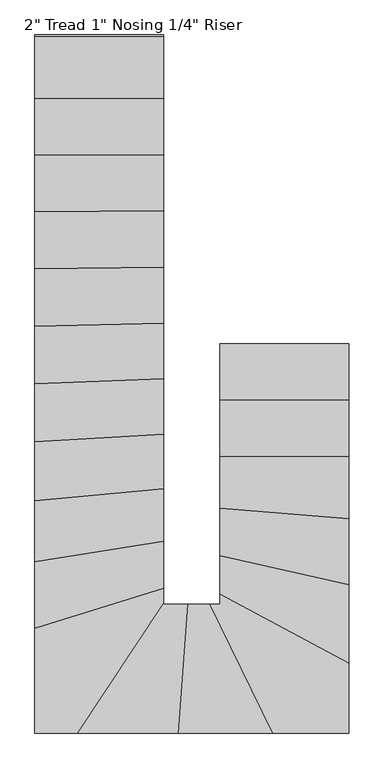
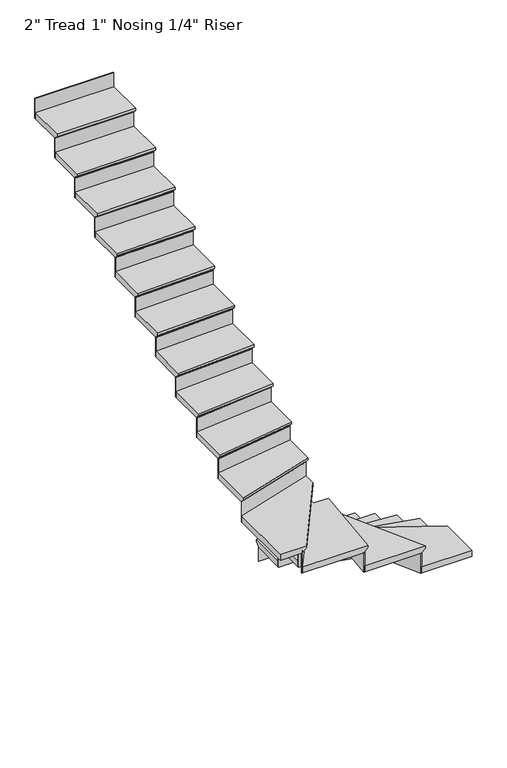
"""IFC4 building model written with IfcOpenShell, lengths in millimetres: stair flight geometry."""

from ifc_helpers import new_model, si_unit, origin, place, context, project, spatial, faceted_brep, source, transform, mapped, element, save


def stair_flight_e7e63c14(model_context):
    return source(origin(), model_context, "Body", "Brep", [
        faceted_brep([(-11643.709927, 2021.0747681, 150.2833333), (-11643.709927, 2021.0747681, 169.3333333), (-11008.709927, 2021.0747681, 169.3333333), (-11008.709927, 2021.0747681, 150.2833333), (-11643.709927, 1995.6747681, 124.8833333), (-11008.709927, 1995.6747681, 124.8833333), (-11643.709927, 1716.2747681, 169.3333333), (-11008.709927, 1716.2747681, 169.3333333), (-11008.709927, 1995.6747681, 118.5333333), (-11008.709927, 1716.2747681, 118.5333333), (-11643.709927, 1716.2747681, 118.5333333), (-11643.709927, 1995.6747681, 118.5333333)], [[[0, 1, 2, 3]], [[4, 0, 3, 5]], [[2, 1, 6, 7]], [[8, 9, 10, 11]], [[2, 7, 9, 8, 5, 3]], [[8, 11, 4, 5]], [[6, 1, 0, 4, 11, 10]], [[7, 6, 10, 9]]]),
        faceted_brep([(-11643.709927, 1995.6747681, 118.5333333), (-11643.709927, 1995.6747681, 0.0), (-11643.709927, 1989.3247681, 0.0), (-11643.709927, 1989.3247681, 118.5333333), (-11008.709927, 1995.6747681, 118.5333333), (-11008.709927, 1989.3247681, 118.5333333), (-11008.709927, 1989.3247681, 0.0), (-11008.709927, 1995.6747681, 0.0)], [[[0, 1, 2, 3]], [[4, 5, 6, 7]], [[1, 0, 4, 7]], [[2, 1, 7, 6]], [[3, 2, 6, 5]], [[0, 3, 5, 4]]]),
        faceted_brep([(-11643.709927, 1716.2747681, 287.8666667), (-11643.709927, 1716.2747681, 118.5333333), (-11643.709927, 1709.9247681, 118.5333333), (-11643.709927, 1709.9247681, 287.8666667), (-11008.709927, 1716.2747681, 287.8666667), (-11008.709927, 1709.9247681, 287.8666667), (-11008.709927, 1709.9247681, 118.5333333), (-11008.709927, 1716.2747681, 118.5333333)], [[[0, 1, 2, 3]], [[4, 5, 6, 7]], [[1, 0, 4, 7]], [[2, 1, 7, 6]], [[3, 2, 6, 5]], [[0, 3, 5, 4]]]),
        faceted_brep([(-11008.709927, 1741.6747681, 338.6666667), (-11643.709927, 1741.6747681, 338.6666667), (-11643.709927, 1436.8747681, 338.6666667), (-11008.709927, 1436.8747681, 338.6666667), (-11008.709927, 1716.2747681, 287.8666667), (-11008.709927, 1436.8747681, 287.8666667), (-11643.709927, 1436.8747681, 287.8666667), (-11643.709927, 1716.2747681, 287.8666667), (-11008.709927, 1716.2747681, 294.2166667), (-11008.709927, 1741.6747681, 319.6166667), (-11643.709927, 1716.2747681, 294.2166667), (-11643.709927, 1741.6747681, 319.6166667)], [[[0, 1, 2, 3]], [[4, 5, 6, 7]], [[0, 3, 5, 4, 8, 9]], [[4, 7, 10, 8]], [[2, 1, 11, 10, 7, 6]], [[3, 2, 6, 5]], [[11, 1, 0, 9]], [[10, 11, 9, 8]]]),
        faceted_brep([(-11643.709927, 1436.8747681, 457.2), (-11643.709927, 1436.8747681, 287.8666667), (-11643.709927, 1430.5247681, 287.8666667), (-11643.709927, 1430.5247681, 457.2), (-11008.709927, 1436.8747681, 457.2), (-11008.709927, 1430.5247681, 457.2), (-11008.709927, 1430.5247681, 287.8666667), (-11008.709927, 1436.8747681, 287.8666667)], [[[0, 1, 2, 3]], [[4, 5, 6, 7]], [[1, 0, 4, 7]], [[2, 1, 7, 6]], [[3, 2, 6, 5]], [[0, 3, 5, 4]]]),
        faceted_brep([(-11008.709927, 1462.2747681, 508.0), (-11643.709927, 1462.2747681, 508.0), (-11643.709927, 1184.2060512, 508.0), (-11008.709927, 1130.5625394, 508.0), (-11008.709927, 1436.8747681, 457.2), (-11008.709927, 1130.5625394, 457.2), (-11643.709927, 1184.2060512, 457.2), (-11643.709927, 1436.8747681, 457.2), (-11008.709927, 1436.8747681, 463.55), (-11008.709927, 1462.2747681, 488.95), (-11643.709927, 1436.8747681, 463.55), (-11643.709927, 1462.2747681, 488.95)], [[[0, 1, 2, 3]], [[4, 5, 6, 7]], [[0, 3, 5, 4, 8, 9]], [[4, 7, 10, 8]], [[2, 1, 11, 10, 7, 6]], [[3, 2, 6, 5]], [[11, 1, 0, 9]], [[10, 11, 9, 8]]]),
        faceted_brep([(-11643.709927, 1184.2060512, 626.5333333), (-11643.709927, 1184.2060512, 457.2), (-11643.709927, 1177.833433, 457.2), (-11643.709927, 1177.833433, 626.5333333), (-11008.709927, 1130.5625394, 626.5333333), (-11008.709927, 1124.1899212, 626.5333333), (-11008.709927, 1124.1899212, 457.2), (-11008.709927, 1130.5625394, 457.2)], [[[0, 1, 2, 3]], [[4, 5, 6, 7]], [[1, 0, 4, 7]], [[2, 1, 7, 6]], [[3, 2, 6, 5]], [[0, 3, 5, 4]]]),
        faceted_brep([(-11008.709927, 1156.0530121, 677.3333333), (-11643.709927, 1209.696524, 677.3333333), (-11643.709927, 949.9239217, 677.3333333), (-11008.709927, 804.9179267, 677.3333333), (-11008.709927, 1130.5625394, 626.5333333), (-11008.709927, 804.9179267, 626.5333333), (-11643.709927, 949.9239217, 626.5333333), (-11643.709927, 1184.2060512, 626.5333333), (-11008.709927, 1130.5625394, 632.8833333), (-11008.709927, 1156.0530121, 658.2833333), (-11643.709927, 1184.2060512, 632.8833333), (-11643.709927, 1209.696524, 658.2833333)], [[[0, 1, 2, 3]], [[4, 5, 6, 7]], [[0, 3, 5, 4, 8, 9]], [[4, 7, 10, 8]], [[2, 1, 11, 10, 7, 6]], [[3, 2, 6, 5]], [[11, 1, 0, 9]], [[10, 11, 9, 8]]]),
        faceted_brep([(-11643.709927, 949.9239217, 795.8666667), (-11643.709927, 949.9239217, 626.5333333), (-11643.709927, 943.4104607, 626.5333333), (-11643.709927, 943.4104607, 795.8666667), (-11008.709927, 804.9179267, 795.8666667), (-11008.709927, 798.4044657, 795.8666667), (-11008.709927, 798.4044657, 626.5333333), (-11008.709927, 804.9179267, 626.5333333)], [[[0, 1, 2, 3]], [[4, 5, 6, 7]], [[1, 0, 4, 7]], [[2, 1, 7, 6]], [[3, 2, 6, 5]], [[0, 3, 5, 4]]]),
        faceted_brep([(-11008.709927, 830.9717706, 846.6666667), (-11643.709927, 975.9777656, 846.6666667), (-11643.709927, 755.0123184, 846.6666667), (-11008.709927, 415.579537, 846.6666667), (-11008.709927, 804.9179267, 795.8666667), (-11008.709927, 415.579537, 795.8666667), (-11643.709927, 755.0123184, 795.8666667), (-11643.709927, 949.9239217, 795.8666667), (-11008.709927, 804.9179267, 802.2166667), (-11008.709927, 830.9717706, 827.6166667), (-11643.709927, 949.9239217, 802.2166667), (-11643.709927, 975.9777656, 827.6166667)], [[[0, 1, 2, 3]], [[4, 5, 6, 7]], [[0, 3, 5, 4, 8, 9]], [[4, 7, 10, 8]], [[2, 1, 11, 10, 7, 6]], [[3, 2, 6, 5]], [[11, 1, 0, 9]], [[10, 11, 9, 8]]]),
        faceted_brep([(-11643.709927, 755.0123184, 965.2), (-11643.709927, 755.0123184, 795.8666667), (-11643.709927, 747.8120433, 795.8666667), (-11643.709927, 747.8120433, 965.2), (-11008.709927, 415.579537, 965.2), (-11008.709927, 408.3792619, 965.2), (-11008.709927, 408.3792619, 795.8666667), (-11008.709927, 415.579537, 795.8666667)], [[[0, 1, 2, 3]], [[4, 5, 6, 7]], [[1, 0, 4, 7]], [[2, 1, 7, 6]], [[3, 2, 6, 5]], [[0, 3, 5, 4]]]),
        faceted_brep([(-11414.9954976, 100.7187882, 1016.0), (-11008.709927, 100.7187882, 1016.0), (-11008.709927, 444.3806373, 1016.0), (-11643.709927, 783.8134188, 1016.0), (-11643.709927, 735.7187882, 1016.0), (-11725.5659587, 735.7187882, 1016.0), (-11008.709927, 100.7187882, 965.2), (-11414.9954976, 100.7187882, 965.2), (-11725.5659587, 735.7187882, 965.2), (-11643.709927, 735.7187882, 965.2), (-11643.709927, 755.0123184, 965.2), (-11008.709927, 415.579537, 965.2), (-11643.709927, 755.0123184, 971.55), (-11008.709927, 415.579537, 971.55), (-11643.709927, 783.8134188, 996.95), (-11008.709927, 444.3806373, 996.95)], [[[0, 1, 2, 3, 4, 5]], [[6, 7, 8, 9, 10, 11]], [[1, 0, 7, 6]], [[11, 10, 12, 13]], [[4, 3, 14, 12, 10, 9]], [[0, 5, 8, 7]], [[14, 3, 2, 15]], [[12, 14, 15, 13]], [[2, 1, 6, 11, 13, 15]], [[5, 4, 9, 8]]]),
        faceted_brep([(-11725.5659587, 735.7187882, 1134.5333333), (-11725.5659587, 735.7187882, 965.2), (-11732.6347564, 735.7187882, 965.2), (-11732.6347564, 735.7187882, 1134.5333333), (-11414.9954976, 100.7187882, 1134.5333333), (-11422.0642953, 100.7187882, 1134.5333333), (-11422.0642953, 100.7187882, 965.2), (-11414.9954976, 100.7187882, 965.2)], [[[0, 1, 2, 3]], [[4, 5, 6, 7]], [[1, 0, 4, 7]], [[2, 1, 7, 6]], [[3, 2, 6, 5]], [[0, 3, 5, 4]]]),
        faceted_brep([(-11386.7203067, 100.7187882, 1185.3333333), (-11697.2907679, 735.7187882, 1185.3333333), (-11831.0692326, 735.7187882, 1185.3333333), (-11876.0424051, 100.7187882, 1185.3333333), (-11414.9954976, 100.7187882, 1134.5333333), (-11876.0424051, 100.7187882, 1134.5333333), (-11831.0692326, 735.7187882, 1134.5333333), (-11725.5659587, 735.7187882, 1134.5333333), (-11414.9954976, 100.7187882, 1140.8833333), (-11386.7203067, 100.7187882, 1166.2833333), (-11725.5659587, 735.7187882, 1140.8833333), (-11697.2907679, 735.7187882, 1166.2833333)], [[[0, 1, 2, 3]], [[4, 5, 6, 7]], [[0, 3, 5, 4, 8, 9]], [[4, 7, 10, 8]], [[2, 1, 11, 10, 7, 6]], [[3, 2, 6, 5]], [[11, 1, 0, 9]], [[10, 11, 9, 8]]]),
        faceted_brep([(-11831.0692326, 735.7187882, 1303.8666667), (-11831.0692326, 735.7187882, 1134.5333333), (-11837.4351385, 735.7187882, 1134.5333333), (-11837.4351385, 735.7187882, 1303.8666667), (-11876.0424051, 100.7187882, 1303.8666667), (-11882.408311, 100.7187882, 1303.8666667), (-11882.408311, 100.7187882, 1134.5333333), (-11876.0424051, 100.7187882, 1134.5333333)], [[[0, 1, 2, 3]], [[4, 5, 6, 7]], [[1, 0, 4, 7]], [[2, 1, 7, 6]], [[3, 2, 6, 5]], [[0, 3, 5, 4]]]),
        faceted_brep([(-11850.5787812, 100.7187882, 1354.6666667), (-11805.6056087, 735.7187882, 1354.6666667), (-11923.109927, 735.7187882, 1354.6666667), (-11923.109927, 789.2110037, 1354.6666667), (-12379.5202352, 100.7187882, 1354.6666667), (-11876.0424051, 100.7187882, 1303.8666667), (-12379.5202352, 100.7187882, 1303.8666667), (-11923.109927, 789.2110037, 1303.8666667), (-11923.109927, 735.7187882, 1303.8666667), (-11831.0692326, 735.7187882, 1303.8666667), (-11876.0424051, 100.7187882, 1310.2166667), (-11850.5787812, 100.7187882, 1335.6166667), (-11831.0692326, 735.7187882, 1310.2166667), (-11805.6056087, 735.7187882, 1335.6166667)], [[[0, 1, 2, 3, 4]], [[5, 6, 7, 8, 9]], [[0, 4, 6, 5, 10, 11]], [[5, 9, 12, 10]], [[3, 2, 8, 7]], [[4, 3, 7, 6]], [[13, 1, 0, 11]], [[12, 13, 11, 10]], [[2, 1, 13, 12, 9, 8]]]),
        faceted_brep([(-11923.109927, 789.2110037, 1473.2), (-11923.109927, 789.2110037, 1303.8666667), (-11923.109927, 800.7035462, 1303.8666667), (-11923.109927, 800.7035462, 1473.2), (-12379.5202352, 100.7187882, 1473.2), (-12387.1387889, 100.7187882, 1473.2), (-12387.1387889, 100.7187882, 1303.8666667), (-12379.5202352, 100.7187882, 1303.8666667)], [[[0, 1, 2, 3]], [[4, 5, 6, 7]], [[1, 0, 4, 7]], [[2, 1, 7, 6]], [[3, 2, 6, 5]], [[0, 3, 5, 4]]]),
        faceted_brep([(-12558.109927, 643.6551613, 1524.0), (-12558.109927, 100.7187882, 1524.0), (-12349.0460207, 100.7187882, 1524.0), (-11923.109927, 743.2408337, 1524.0), (-11923.109927, 841.8492807, 1524.0), (-12558.109927, 100.7187882, 1473.2), (-12558.109927, 643.6551613, 1473.2), (-11923.109927, 841.8492807, 1473.2), (-11923.109927, 789.2110037, 1473.2), (-12379.5202352, 100.7187882, 1473.2), (-11923.109927, 789.2110037, 1479.55), (-12379.5202352, 100.7187882, 1479.55), (-11923.109927, 743.2408337, 1504.95), (-12349.0460207, 100.7187882, 1504.95)], [[[0, 1, 2, 3, 4]], [[5, 6, 7, 8, 9]], [[1, 0, 6, 5]], [[9, 8, 10, 11]], [[4, 3, 12, 10, 8, 7]], [[0, 4, 7, 6]], [[12, 3, 2, 13]], [[10, 12, 13, 11]], [[2, 1, 5, 9, 11, 13]]]),
        faceted_brep([(-11923.109927, 841.8492807, 1642.5333333), (-11923.109927, 841.8492807, 1473.2), (-11923.109927, 848.5013925, 1473.2), (-11923.109927, 848.5013925, 1642.5333333), (-12558.109927, 643.6551613, 1642.5333333), (-12558.109927, 650.3072731, 1642.5333333), (-12558.109927, 650.3072731, 1473.2), (-12558.109927, 643.6551613, 1473.2)], [[[0, 1, 2, 3]], [[4, 5, 6, 7]], [[1, 0, 4, 7]], [[2, 1, 7, 6]], [[3, 2, 6, 5]], [[0, 3, 5, 4]]]),
        faceted_brep([(-12558.109927, 617.0467142, 1693.3333333), (-11923.109927, 815.2408337, 1693.3333333), (-11923.109927, 1070.9435536, 1693.3333333), (-12558.109927, 971.92657, 1693.3333333), (-12558.109927, 643.6551613, 1642.5333333), (-12558.109927, 971.92657, 1642.5333333), (-11923.109927, 1070.9435536, 1642.5333333), (-11923.109927, 841.8492807, 1642.5333333), (-12558.109927, 643.6551613, 1648.8833333), (-12558.109927, 617.0467142, 1674.2833333), (-11923.109927, 841.8492807, 1648.8833333), (-11923.109927, 815.2408337, 1674.2833333)], [[[0, 1, 2, 3]], [[4, 5, 6, 7]], [[0, 3, 5, 4, 8, 9]], [[4, 7, 10, 8]], [[2, 1, 11, 10, 7, 6]], [[3, 2, 6, 5]], [[11, 1, 0, 9]], [[10, 11, 9, 8]]]),
        faceted_brep([(-11923.109927, 1070.9435536, 1811.8666667), (-11923.109927, 1070.9435536, 1642.5333333), (-11923.109927, 1077.3702896, 1642.5333333), (-11923.109927, 1077.3702896, 1811.8666667), (-12558.109927, 971.92657, 1811.8666667), (-12558.109927, 978.3533061, 1811.8666667), (-12558.109927, 978.3533061, 1642.5333333), (-12558.109927, 971.92657, 1642.5333333)], [[[0, 1, 2, 3]], [[4, 5, 6, 7]], [[1, 0, 4, 7]], [[2, 1, 7, 6]], [[3, 2, 6, 5]], [[0, 3, 5, 4]]]),
        faceted_brep([(-12558.109927, 946.2196258, 1862.6666667), (-11923.109927, 1045.2366094, 1862.6666667), (-11923.109927, 1330.3354541, 1862.6666667), (-12558.109927, 1270.9425034, 1862.6666667), (-12558.109927, 971.92657, 1811.8666667), (-12558.109927, 1270.9425034, 1811.8666667), (-11923.109927, 1330.3354541, 1811.8666667), (-11923.109927, 1070.9435536, 1811.8666667), (-12558.109927, 971.92657, 1818.2166667), (-12558.109927, 946.2196258, 1843.6166667), (-11923.109927, 1070.9435536, 1818.2166667), (-11923.109927, 1045.2366094, 1843.6166667)], [[[0, 1, 2, 3]], [[4, 5, 6, 7]], [[0, 3, 5, 4, 8, 9]], [[4, 7, 10, 8]], [[2, 1, 11, 10, 7, 6]], [[3, 2, 6, 5]], [[11, 1, 0, 9]], [[10, 11, 9, 8]]]),
        faceted_brep([(-11923.109927, 1330.3354541, 1981.2), (-11923.109927, 1330.3354541, 1811.8666667), (-11923.109927, 1336.7131694, 1811.8666667), (-11923.109927, 1336.7131694, 1981.2), (-12558.109927, 1270.9425034, 1981.2), (-12558.109927, 1277.3202186, 1981.2), (-12558.109927, 1277.3202186, 1811.8666667), (-12558.109927, 1270.9425034, 1811.8666667)], [[[0, 1, 2, 3]], [[4, 5, 6, 7]], [[1, 0, 4, 7]], [[2, 1, 7, 6]], [[3, 2, 6, 5]], [[0, 3, 5, 4]]]),
        faceted_brep([(-12558.109927, 1245.4316422, 2032.0), (-11923.109927, 1304.8245929, 2032.0), (-11923.109927, 1599.0069444, 2032.0), (-12558.109927, 1560.9404879, 2032.0), (-12558.109927, 1270.9425034, 1981.2), (-12558.109927, 1560.9404879, 1981.2), (-11923.109927, 1599.0069444, 1981.2), (-11923.109927, 1330.3354541, 1981.2), (-12558.109927, 1270.9425034, 1987.55), (-12558.109927, 1245.4316422, 2012.95), (-11923.109927, 1330.3354541, 1987.55), (-11923.109927, 1304.8245929, 2012.95)], [[[0, 1, 2, 3]], [[4, 5, 6, 7]], [[0, 3, 5, 4, 8, 9]], [[4, 7, 10, 8]], [[2, 1, 11, 10, 7, 6]], [[3, 2, 6, 5]], [[11, 1, 0, 9]], [[10, 11, 9, 8]]]),
        faceted_brep([(-11923.109927, 1599.0069444, 2150.5333333), (-11923.109927, 1599.0069444, 1981.2), (-11923.109927, 1605.3683441, 1981.2), (-11923.109927, 1605.3683441, 2150.5333333), (-12558.109927, 1560.9404879, 2150.5333333), (-12558.109927, 1567.3018876, 2150.5333333), (-12558.109927, 1567.3018876, 1981.2), (-12558.109927, 1560.9404879, 1981.2)], [[[0, 1, 2, 3]], [[4, 5, 6, 7]], [[1, 0, 4, 7]], [[2, 1, 7, 6]], [[3, 2, 6, 5]], [[0, 3, 5, 4]]]),
        faceted_brep([(-12558.109927, 1535.4948893, 2201.3333333), (-11923.109927, 1573.5613458, 2201.3333333), (-11923.109927, 1871.7177797, 2201.3333333), (-12558.109927, 1846.9769987, 2201.3333333), (-12558.109927, 1560.9404879, 2150.5333333), (-12558.109927, 1846.9769987, 2150.5333333), (-11923.109927, 1871.7177797, 2150.5333333), (-11923.109927, 1599.0069444, 2150.5333333), (-12558.109927, 1560.9404879, 2156.8833333), (-12558.109927, 1535.4948893, 2182.2833333), (-11923.109927, 1599.0069444, 2156.8833333), (-11923.109927, 1573.5613458, 2182.2833333)], [[[0, 1, 2, 3]], [[4, 5, 6, 7]], [[0, 3, 5, 4, 8, 9]], [[4, 7, 10, 8]], [[2, 1, 11, 10, 7, 6]], [[3, 2, 6, 5]], [[11, 1, 0, 9]], [[10, 11, 9, 8]]]),
        faceted_brep([(-11923.109927, 1871.7177797, 2319.8666667), (-11923.109927, 1871.7177797, 2150.5333333), (-11923.109927, 1878.0725976, 2150.5333333), (-11923.109927, 1878.0725976, 2319.8666667), (-12558.109927, 1846.9769987, 2319.8666667), (-12558.109927, 1853.3318166, 2319.8666667), (-12558.109927, 1853.3318166, 2150.5333333), (-12558.109927, 1846.9769987, 2150.5333333)], [[[0, 1, 2, 3]], [[4, 5, 6, 7]], [[1, 0, 4, 7]], [[2, 1, 7, 6]], [[3, 2, 6, 5]], [[0, 3, 5, 4]]]),
        faceted_brep([(-12558.109927, 1821.5577271, 2370.6666667), (-11923.109927, 1846.2985081, 2370.6666667), (-11923.109927, 2146.5481619, 2370.6666667), (-12558.109927, 2130.9234493, 2370.6666667), (-12558.109927, 1846.9769987, 2319.8666667), (-12558.109927, 2130.9234493, 2319.8666667), (-11923.109927, 2146.5481619, 2319.8666667), (-11923.109927, 1871.7177797, 2319.8666667), (-12558.109927, 1846.9769987, 2326.2166667), (-12558.109927, 1821.5577271, 2351.6166667), (-11923.109927, 1871.7177797, 2326.2166667), (-11923.109927, 1846.2985081, 2351.6166667)], [[[0, 1, 2, 3]], [[4, 5, 6, 7]], [[0, 3, 5, 4, 8, 9]], [[4, 7, 10, 8]], [[2, 1, 11, 10, 7, 6]], [[3, 2, 6, 5]], [[11, 1, 0, 9]], [[10, 11, 9, 8]]]),
        faceted_brep([(-11923.109927, 2146.5481619, 2489.2), (-11923.109927, 2146.5481619, 2319.8666667), (-11923.109927, 2152.900084, 2319.8666667), (-11923.109927, 2152.900084, 2489.2), (-12558.109927, 2130.9234493, 2489.2), (-12558.109927, 2137.2753713, 2489.2), (-12558.109927, 2137.2753713, 2319.8666667), (-12558.109927, 2130.9234493, 2319.8666667)], [[[0, 1, 2, 3]], [[4, 5, 6, 7]], [[1, 0, 4, 7]], [[2, 1, 7, 6]], [[3, 2, 6, 5]], [[0, 3, 5, 4]]]),
        faceted_brep([(-12558.109927, 2105.5157612, 2540.0), (-11923.109927, 2121.1404739, 2540.0), (-11923.109927, 2422.628471, 2540.0), (-12558.109927, 2413.6328613, 2540.0), (-12558.109927, 2130.9234493, 2489.2), (-12558.109927, 2413.6328613, 2489.2), (-11923.109927, 2422.628471, 2489.2), (-11923.109927, 2146.5481619, 2489.2), (-12558.109927, 2130.9234493, 2495.55), (-12558.109927, 2105.5157612, 2520.95), (-11923.109927, 2146.5481619, 2495.55), (-11923.109927, 2121.1404739, 2520.95)], [[[0, 1, 2, 3]], [[4, 5, 6, 7]], [[0, 3, 5, 4, 8, 9]], [[4, 7, 10, 8]], [[2, 1, 11, 10, 7, 6]], [[3, 2, 6, 5]], [[11, 1, 0, 9]], [[10, 11, 9, 8]]]),
        faceted_brep([(-11923.109927, 2422.628471, 2658.5333333), (-11923.109927, 2422.628471, 2489.2), (-11923.109927, 2428.9791081, 2489.2), (-11923.109927, 2428.9791081, 2658.5333333), (-12558.109927, 2413.6328613, 2658.5333333), (-12558.109927, 2419.9834984, 2658.5333333), (-12558.109927, 2419.9834984, 2489.2), (-12558.109927, 2413.6328613, 2489.2)], [[[0, 1, 2, 3]], [[4, 5, 6, 7]], [[1, 0, 4, 7]], [[2, 1, 7, 6]], [[3, 2, 6, 5]], [[0, 3, 5, 4]]]),
        faceted_brep([(-12558.109927, 2388.2303127, 2709.3333333), (-11923.109927, 2397.2259224, 2709.3333333), (-11923.109927, 2699.507572, 2709.3333333), (-12558.109927, 2695.5496499, 2709.3333333), (-12558.109927, 2413.6328613, 2658.5333333), (-12558.109927, 2695.5496499, 2658.5333333), (-11923.109927, 2699.507572, 2658.5333333), (-11923.109927, 2422.628471, 2658.5333333), (-12558.109927, 2413.6328613, 2664.8833333), (-12558.109927, 2388.2303127, 2690.2833333), (-11923.109927, 2422.628471, 2664.8833333), (-11923.109927, 2397.2259224, 2690.2833333)], [[[0, 1, 2, 3]], [[4, 5, 6, 7]], [[0, 3, 5, 4, 8, 9]], [[4, 7, 10, 8]], [[2, 1, 11, 10, 7, 6]], [[3, 2, 6, 5]], [[11, 1, 0, 9]], [[10, 11, 9, 8]]]),
        faceted_brep([(-11923.109927, 2699.507572, 2827.8666667), (-11923.109927, 2699.507572, 2658.5333333), (-11923.109927, 2705.8576954, 2658.5333333), (-11923.109927, 2705.8576954, 2827.8666667), (-12558.109927, 2695.5496499, 2827.8666667), (-12558.109927, 2701.8997732, 2827.8666667), (-12558.109927, 2701.8997732, 2658.5333333), (-12558.109927, 2695.5496499, 2658.5333333)], [[[0, 1, 2, 3]], [[4, 5, 6, 7]], [[1, 0, 4, 7]], [[2, 1, 7, 6]], [[3, 2, 6, 5]], [[0, 3, 5, 4]]]),
        faceted_brep([(-12558.109927, 2670.1491565, 2878.6666667), (-11923.109927, 2674.1070787, 2878.6666667), (-11923.109927, 2976.9281176, 2878.6666667), (-12558.109927, 2976.9281176, 2878.6666667), (-12558.109927, 2695.5496499, 2827.8666667), (-12558.109927, 2976.9281176, 2827.8666667), (-11923.109927, 2976.9281176, 2827.8666667), (-11923.109927, 2699.507572, 2827.8666667), (-12558.109927, 2695.5496499, 2834.2166667), (-12558.109927, 2670.1491565, 2859.6166667), (-11923.109927, 2699.507572, 2834.2166667), (-11923.109927, 2674.1070787, 2859.6166667)], [[[0, 1, 2, 3]], [[4, 5, 6, 7]], [[0, 3, 5, 4, 8, 9]], [[4, 7, 10, 8]], [[2, 1, 11, 10, 7, 6]], [[3, 2, 6, 5]], [[11, 1, 0, 9]], [[10, 11, 9, 8]]]),
        faceted_brep([(-11923.109927, 2976.9281176, 2997.2), (-11923.109927, 2976.9281176, 2827.8666667), (-11923.109927, 2983.2781176, 2827.8666667), (-11923.109927, 2983.2781176, 2997.2), (-12558.109927, 2976.9281176, 2997.2), (-12558.109927, 2983.2781176, 2997.2), (-12558.109927, 2983.2781176, 2827.8666667), (-12558.109927, 2976.9281176, 2827.8666667)], [[[0, 1, 2, 3]], [[4, 5, 6, 7]], [[1, 0, 4, 7]], [[2, 1, 7, 6]], [[3, 2, 6, 5]], [[0, 3, 5, 4]]]),
        faceted_brep([(-12558.109927, 2951.5281176, 3048.0), (-11923.109927, 2951.5281176, 3048.0), (-11923.109927, 3256.3281176, 3048.0), (-12558.109927, 3256.3281176, 3048.0), (-12558.109927, 2976.9281176, 2997.2), (-12558.109927, 3256.3281176, 2997.2), (-11923.109927, 3256.3281176, 2997.2), (-11923.109927, 2976.9281176, 2997.2), (-12558.109927, 2976.9281176, 3003.55), (-12558.109927, 2951.5281176, 3028.95), (-11923.109927, 2976.9281176, 3003.55), (-11923.109927, 2951.5281176, 3028.95)], [[[0, 1, 2, 3]], [[4, 5, 6, 7]], [[0, 3, 5, 4, 8, 9]], [[4, 7, 10, 8]], [[2, 1, 11, 10, 7, 6]], [[3, 2, 6, 5]], [[11, 1, 0, 9]], [[10, 11, 9, 8]]]),
        faceted_brep([(-11923.109927, 3256.3281176, 3166.5333333), (-11923.109927, 3256.3281176, 2997.2), (-11923.109927, 3262.6781176, 2997.2), (-11923.109927, 3262.6781176, 3166.5333333), (-12558.109927, 3256.3281176, 3166.5333333), (-12558.109927, 3262.6781176, 3166.5333333), (-12558.109927, 3262.6781176, 2997.2), (-12558.109927, 3256.3281176, 2997.2)], [[[0, 1, 2, 3]], [[4, 5, 6, 7]], [[1, 0, 4, 7]], [[2, 1, 7, 6]], [[3, 2, 6, 5]], [[0, 3, 5, 4]]]),
        faceted_brep([(-11923.109927, 3535.7281176, 3335.8666667), (-11923.109927, 3535.7281176, 3166.5333333), (-11923.109927, 3542.0781176, 3166.5333333), (-11923.109927, 3542.0781176, 3335.8666667), (-12558.109927, 3535.7281176, 3335.8666667), (-12558.109927, 3542.0781176, 3335.8666667), (-12558.109927, 3542.0781176, 3166.5333333), (-12558.109927, 3535.7281176, 3166.5333333)], [[[0, 1, 2, 3]], [[4, 5, 6, 7]], [[1, 0, 4, 7]], [[2, 1, 7, 6]], [[3, 2, 6, 5]], [[0, 3, 5, 4]]]),
        faceted_brep([(-12558.109927, 3230.9281176, 3217.3333333), (-11923.109927, 3230.9281176, 3217.3333333), (-11923.109927, 3535.7281176, 3217.3333333), (-12558.109927, 3535.7281176, 3217.3333333), (-12558.109927, 3256.3281176, 3166.5333333), (-12558.109927, 3535.7281176, 3166.5333333), (-11923.109927, 3535.7281176, 3166.5333333), (-11923.109927, 3256.3281176, 3166.5333333), (-12558.109927, 3256.3281176, 3172.8833333), (-12558.109927, 3230.9281176, 3198.2833333), (-11923.109927, 3256.3281176, 3172.8833333), (-11923.109927, 3230.9281176, 3198.2833333)], [[[0, 1, 2, 3]], [[4, 5, 6, 7]], [[0, 3, 5, 4, 8, 9]], [[4, 7, 10, 8]], [[2, 1, 11, 10, 7, 6]], [[3, 2, 6, 5]], [[11, 1, 0, 9]], [[10, 11, 9, 8]]]),
    ])


if __name__ == "__main__":
    model = new_model("IFC4")
    model_context = context("Model", 3, world=origin())
    ifc_project = project(units=[si_unit("LENGTHUNIT", "METRE", prefix="MILLI")], contexts=[model_context])
    site = spatial("IfcSite", under=ifc_project)
    building = spatial("IfcBuilding", under=site)
    placement = place(None, origin())
    stair_flight_shape = stair_flight_e7e63c14(model_context)
    element("IfcStairFlight", 1, ObjectType="2\" Tread 1\" Nosing 1/4\" Riser", at=placement, inside=building, context=model_context, shape_type="MappedRepresentation", body=[
        mapped(stair_flight_shape, transform((0.0, 0.0, 0.0), x_axis=(1.0, 0.0, 0.0), y_axis=(0.0, 1.0, 0.0), z_axis=(0.0, 0.0, 1.0))),
    ])
    save(model, "model.ifc")
